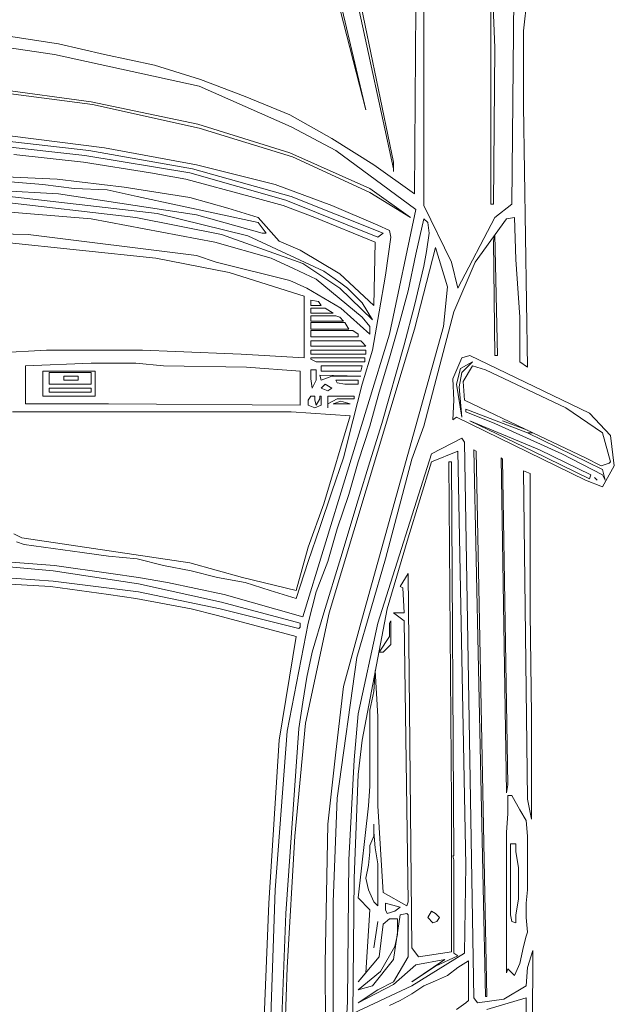
# Model space of a CAD drawing. Units: inches. Extents: x -36302355 to 648, y -221479757 to 75.
# Tile 9 of 37: x 209 to 227, y -484 to -455. Entities that reach past the tile are written whole.
import ezdxf

# ---------------------------------------------------------------- set-up
doc = ezdxf.new("R2010")
doc.units = ezdxf.units.IN
doc.header["$MEASUREMENT"] = 0
doc.layers.add('A-EQPM-VEHC', color=8, linetype='Continuous', lineweight=13)

msp = doc.modelspace()

# ---------------------------------------------------------------- linework, layer by layer
at = {"layer": 'A-EQPM-VEHC'}
for p, q in [((216.133, -443.293), (219.515, -457.606)), ((223.014, -446.517), (223.368, -455.758)), ((220.341, -459.375), (217.667, -447.067)), ((221.245, -447.264), (221.245, -460.477)), ((218.178, -448.798), (220.341, -459.178)), ((223.879, -460.437), (223.958, -452.847)), ((219.515, -457.606), (218.374, -453.163)), ((224.233, -455.246), (224.351, -454.146)), ((220.969, -460.122), (221.01, -454.539)), ((223.25, -460.437), (223.25, -454.618)), ((224.233, -457.489), (224.233, -455.246)), ((210.195, -455.955), (207.207, -455.522)), ((208.818, -455.404), (210.313, -455.639)), ((210.313, -455.639), (211.689, -455.955)), ((223.368, -455.758), (223.329, -460.437)), ((214.521, -456.899), (210.195, -455.955)), ((211.689, -455.955), (213.184, -456.269)), ((213.184, -456.269), (214.559, -456.701)), ((214.559, -456.701), (215.897, -457.213)), ((207.679, -456.976), (211.336, -457.448)), ((211.296, -457.369), (207.797, -456.899)), ((217.274, -458.117), (214.521, -456.899)), ((214.481, -458.038), (211.296, -457.369)), ((215.897, -457.213), (217.234, -457.764)), ((211.336, -457.448), (214.521, -458.157)), ((224.351, -465.313), (224.233, -457.489)), ((217.234, -457.764), (218.492, -458.471)), ((217.234, -458.903), (214.481, -458.038)), ((214.521, -458.157), (217.313, -459.022)), ((218.611, -458.826), (217.274, -458.117)), ((211.217, -458.826), (208.072, -458.471)), ((211.689, -458.747), (208.858, -458.392)), ((218.492, -458.471), (219.75, -459.257)), ((207.993, -458.629), (211.099, -458.982)), ((214.324, -459.375), (211.217, -458.826)), ((214.442, -459.257), (211.689, -458.747)), ((221.01, -460.594), (218.611, -458.826)), ((211.06, -459.178), (208.976, -458.943)), ((213.066, -459.494), (211.06, -459.178)), ((211.099, -458.982), (214.245, -459.494)), ((219.632, -459.966), (217.234, -458.903)), ((217.313, -459.022), (219.632, -460.084)), ((220.341, -459.178), (220.341, -459.454)), ((204.021, -459.375), (210.274, -459.691)), ((217.274, -460.201), (214.324, -459.375)), ((216.802, -459.847), (214.442, -459.257)), ((219.75, -459.257), (220.969, -460.122)), ((209.841, -459.847), (207.953, -459.691)), ((210.274, -459.691), (212.28, -459.926)), ((214.128, -459.691), (213.066, -459.494)), ((216.054, -460.201), (214.128, -459.691)), ((214.245, -459.494), (217.116, -460.319)), ((204.689, -459.808), (210.313, -460.122)), ((210.785, -459.966), (209.841, -459.847)), ((211.768, -460.005), (210.785, -459.966)), ((212.673, -460.201), (211.768, -460.005)), ((212.28, -459.926), (214.245, -460.24)), ((218.492, -460.477), (216.802, -459.847)), ((220.852, -460.831), (219.632, -459.966)), ((213.263, -460.712), (208.111, -460.122)), ((208.228, -460.319), (212.633, -460.831)), ((210.313, -460.122), (214.442, -460.752)), ((216.29, -460.988), (212.673, -460.201)), ((214.245, -460.24), (215.386, -460.556)), ((217.037, -460.477), (216.054, -460.201)), ((217.116, -460.319), (219.869, -461.421)), ((220.025, -461.302), (217.274, -460.201)), ((219.632, -460.084), (220.852, -460.831)), ((211.296, -460.87), (207.483, -460.556)), ((215.386, -460.556), (216.29, -460.831)), ((217.981, -460.831), (217.037, -460.477)), ((219.869, -461.066), (218.492, -460.477)), ((220.222, -464.33), (221.01, -460.594)), ((221.245, -460.477), (222.071, -462.167)), ((223.329, -460.437), (223.25, -460.437)), ((223.368, -460.831), (223.879, -460.437)), ((214.993, -461.577), (211.296, -460.87)), ((212.633, -460.831), (215.189, -461.342)), ((215.975, -461.381), (213.263, -460.712)), ((214.442, -460.752), (216.409, -461.302)), ((216.29, -460.831), (216.919, -461.538)), ((219.79, -461.577), (217.981, -460.831)), ((221.245, -460.87), (221.01, -461.932)), ((221.362, -460.988), (221.245, -460.87)), ((222.268, -462.954), (223.368, -460.831)), ((222.778, -462.167), (223.722, -460.87)), ((223.722, -460.87), (223.958, -460.831)), ((223.958, -460.831), (223.998, -462.089)), ((216.526, -461.302), (216.29, -460.988)), ((220.222, -461.224), (219.869, -461.066)), ((220.262, -461.421), (220.222, -461.224)), ((221.403, -461.302), (221.362, -460.988)), ((207.679, -461.302), (209.409, -461.342)), ((209.409, -461.342), (214.442, -461.97)), ((215.189, -461.342), (217.627, -462.207)), ((218.257, -462.442), (215.975, -461.381)), ((216.409, -461.302), (216.526, -461.302)), ((216.919, -461.538), (217.548, -461.814)), ((219.869, -461.421), (220.025, -461.302)), ((220.104, -462.561), (220.262, -461.421)), ((221.324, -461.853), (221.403, -461.302)), ((223.368, -461.342), (223.329, -461.538)), ((223.329, -461.538), (223.368, -464.96)), ((223.447, -464.96), (223.368, -461.342)), ((213.222, -462.049), (208.662, -461.577)), ((216.683, -462.049), (214.993, -461.577)), ((217.548, -461.814), (218.729, -462.521)), ((219.75, -463.465), (219.79, -461.577)), ((220.969, -464.172), (221.599, -461.735)), ((221.599, -461.735), (221.952, -462.914)), ((215.425, -462.482), (213.222, -462.049)), ((214.442, -461.97), (215.031, -462.167)), ((217.351, -462.365), (216.683, -462.049)), ((221.01, -461.932), (220.773, -463.032)), ((221.245, -462.286), (221.324, -461.853)), ((223.998, -462.089), (224.116, -463.82)), ((215.031, -462.167), (217.234, -462.718)), ((218.02, -462.679), (217.351, -462.365)), ((217.627, -462.207), (218.729, -462.954)), ((220.969, -463.465), (221.245, -462.286)), ((222.071, -462.167), (222.268, -462.954)), ((222.149, -463.662), (222.778, -462.167)), ((217.667, -463.19), (215.425, -462.482)), ((217.234, -462.718), (217.746, -462.954)), ((219.397, -463.82), (218.02, -462.679)), ((218.767, -462.797), (218.257, -462.442)), ((218.729, -462.521), (219.75, -463.465)), ((219.908, -463.662), (220.104, -462.561)), ((217.746, -462.954), (218.767, -463.544)), ((218.729, -462.954), (219.711, -463.898)), ((218.964, -462.954), (218.767, -462.797)), ((219.397, -463.386), (218.964, -462.954)), ((221.952, -462.914), (221.834, -464.095)), ((217.667, -465.037), (217.667, -463.19)), ((218.099, -463.348), (217.863, -463.307)), ((217.863, -463.307), (217.863, -463.465)), ((220.773, -463.032), (220.497, -464.055)), ((217.863, -463.465), (218.178, -463.465)), ((218.295, -463.544), (217.863, -463.544)), ((217.863, -463.544), (217.863, -463.7)), ((218.178, -463.465), (218.099, -463.348)), ((218.532, -463.7), (218.295, -463.544)), ((218.767, -463.544), (219.632, -464.33)), ((219.711, -463.898), (219.397, -463.386)), ((220.655, -464.644), (220.969, -463.465)), ((217.863, -463.7), (218.532, -463.7)), ((218.611, -463.779), (217.863, -463.779)), ((217.863, -463.779), (217.863, -463.937)), ((218.729, -463.82), (218.611, -463.779)), ((218.846, -463.937), (218.729, -463.82)), ((219.632, -464.095), (219.397, -463.82)), ((219.711, -464.802), (219.908, -463.662)), ((221.245, -467.083), (222.149, -463.662)), ((224.116, -463.82), (224.116, -465.157)), ((217.863, -463.937), (218.846, -463.937)), ((218.885, -463.976), (217.863, -463.976)), ((217.863, -463.976), (217.863, -464.172)), ((217.863, -464.172), (219.004, -464.172)), ((218.413, -472.667), (220.969, -464.172)), ((219.004, -464.172), (218.885, -463.976)), ((221.834, -464.095), (219.357, -472.981)), ((219.632, -464.33), (219.632, -464.095)), ((220.497, -464.055), (220.222, -465.037)), ((217.627, -472.784), (220.222, -464.33)), ((219.122, -464.213), (217.863, -464.213)), ((217.863, -464.213), (217.863, -464.409)), ((217.863, -464.409), (219.279, -464.409)), ((219.279, -464.33), (219.122, -464.213)), ((219.279, -464.409), (219.279, -464.33)), ((219.357, -464.527), (217.863, -464.527)), ((217.863, -464.527), (217.863, -464.685)), ((217.863, -464.685), (219.515, -464.685)), ((219.397, -464.565), (219.357, -464.527)), ((219.515, -464.685), (219.397, -464.565)), ((219.987, -467.004), (220.655, -464.644)), ((207.993, -464.92), (209.959, -464.802)), ((209.959, -464.802), (212.829, -464.802)), ((212.829, -464.802), (213.814, -464.841)), ((213.814, -464.841), (215.779, -464.92)), ((215.779, -464.92), (217.667, -465.037)), ((219.515, -464.802), (217.863, -464.802)), ((217.863, -464.802), (217.863, -464.92)), ((217.863, -464.92), (219.515, -464.92)), ((219.476, -465.037), (217.863, -465.037)), ((217.863, -465.037), (217.863, -465.078)), ((217.863, -465.078), (218.02, -465.157)), ((219.397, -465.825), (219.711, -464.802)), ((219.476, -465.157), (219.476, -465.037)), ((219.515, -464.92), (219.515, -464.802)), ((220.222, -465.037), (219.908, -466.06)), ((222.385, -465.037), (222.11, -465.667)), ((222.621, -464.96), (222.385, -465.037)), ((226.2, -466.69), (222.621, -464.96)), ((223.368, -464.96), (223.447, -464.96)), ((211.296, -465.195), (209.33, -465.274)), ((209.33, -465.274), (209.33, -466.415)), ((212.633, -465.195), (211.296, -465.195)), ((213.459, -465.274), (212.633, -465.195)), ((215.937, -465.313), (213.459, -465.274)), ((217.548, -465.431), (215.937, -465.313)), ((218.02, -465.157), (219.476, -465.157)), ((219.397, -465.274), (218.178, -465.274)), ((218.178, -465.274), (218.178, -465.431)), ((219.357, -465.431), (219.397, -465.274)), ((222.345, -465.353), (222.228, -465.825)), ((222.7, -465.157), (222.345, -465.353)), ((222.385, -465.471), (222.7, -465.157)), ((222.7, -465.274), (222.424, -465.746)), ((223.093, -465.392), (222.7, -465.274)), ((224.116, -465.157), (224.351, -465.313)), ((211.415, -465.431), (209.841, -465.431)), ((209.841, -465.431), (209.841, -466.178)), ((211.296, -465.471), (210.038, -465.471)), ((210.038, -465.471), (210.038, -465.825)), ((210.903, -465.588), (210.471, -465.588)), ((210.471, -465.588), (210.471, -465.706)), ((210.903, -465.706), (210.903, -465.588)), ((211.296, -465.825), (211.296, -465.471)), ((211.415, -466.178), (211.415, -465.431)), ((217.548, -466.453), (217.548, -465.431)), ((218.02, -465.392), (217.863, -465.392)), ((217.863, -465.392), (217.863, -465.667)), ((217.863, -465.667), (217.902, -465.943)), ((218.02, -465.706), (218.02, -465.392)), ((219.357, -465.588), (218.139, -465.55)), ((218.139, -465.55), (218.178, -465.706)), ((218.178, -465.431), (219.357, -465.431)), ((218.178, -465.706), (218.492, -465.588)), ((218.492, -465.588), (219.357, -465.588)), ((222.11, -465.667), (222.149, -466.297)), ((222.306, -465.903), (222.385, -465.471)), ((225.491, -466.532), (223.093, -465.392)), ((210.038, -465.825), (211.296, -465.825)), ((211.296, -465.943), (210.038, -465.943)), ((210.038, -465.943), (210.038, -466.06)), ((210.471, -465.706), (210.903, -465.706)), ((211.296, -466.06), (211.296, -465.943)), ((217.902, -465.943), (218.02, -465.706)), ((218.295, -465.825), (218.178, -465.943)), ((218.178, -465.943), (218.374, -466.022)), ((218.492, -465.943), (218.295, -465.825)), ((218.374, -466.022), (218.492, -465.943)), ((219.279, -465.706), (218.611, -465.706)), ((218.611, -465.706), (218.65, -465.785)), ((218.65, -465.785), (218.885, -465.825)), ((218.885, -465.825), (219.279, -465.825)), ((219.122, -466.925), (219.397, -465.825)), ((219.279, -465.825), (219.279, -465.706)), ((222.228, -465.825), (222.385, -466.808)), ((222.385, -466.808), (222.306, -465.903)), ((222.424, -465.746), (222.464, -466.297)), ((209.841, -466.178), (211.415, -466.178)), ((210.038, -466.06), (211.296, -466.06)), ((217.863, -466.178), (217.785, -466.297)), ((217.981, -466.178), (217.863, -466.178)), ((217.981, -466.297), (217.981, -466.178)), ((218.139, -466.257), (218.02, -466.453)), ((218.178, -466.178), (218.139, -466.178)), ((218.139, -466.178), (218.139, -466.257)), ((218.178, -466.453), (218.178, -466.178)), ((219.16, -466.178), (218.374, -466.178)), ((218.374, -466.178), (218.374, -466.532)), ((218.374, -466.415), (218.65, -466.257)), ((218.65, -466.257), (219.16, -466.257)), ((219.16, -466.257), (219.16, -466.178)), ((219.908, -466.06), (219.632, -467.083)), ((209.33, -466.415), (211.808, -466.415)), ((211.808, -466.415), (217.548, -466.453)), ((217.785, -466.297), (217.785, -466.453)), ((217.785, -466.453), (217.981, -466.532)), ((218.02, -466.453), (217.981, -466.297)), ((217.981, -466.532), (218.178, -466.453)), ((218.767, -466.336), (218.532, -466.415)), ((218.532, -466.415), (219.043, -466.415)), ((219.043, -466.415), (218.767, -466.336)), ((222.149, -466.297), (222.11, -466.887)), ((222.464, -466.297), (224.509, -467.28)), ((226.593, -467.28), (225.491, -466.532)), ((217.274, -466.65), (208.937, -466.65)), ((219.043, -466.768), (217.274, -466.65)), ((218.257, -469.403), (219.043, -466.768)), ((222.11, -466.887), (222.228, -466.808)), ((222.228, -466.808), (226.081, -468.696)), ((224.351, -467.28), (222.503, -466.571)), ((222.503, -466.571), (222.503, -466.65)), ((222.503, -466.65), (223.368, -467.004)), ((226.828, -467.359), (226.2, -466.69)), ((218.846, -468.027), (219.122, -466.925)), ((219.632, -467.083), (219.279, -468.145)), ((219.632, -468.145), (219.987, -467.004)), ((220.89, -468.066), (221.245, -467.083)), ((222.621, -466.925), (224.509, -467.831)), ((224.705, -467.791), (222.621, -466.925)), ((223.368, -467.004), (225.374, -467.908)), ((223.605, -466.925), (224.351, -467.201)), ((222.385, -467.436), (221.48, -467.908)), ((222.464, -467.555), (222.385, -467.436)), ((226.593, -468.38), (224.351, -467.28)), ((224.351, -467.28), (224.509, -467.28)), ((224.509, -467.28), (226.081, -468.027)), ((226.828, -468.145), (226.593, -467.28)), ((226.946, -468.263), (226.828, -467.359)), ((222.74, -484.188), (222.464, -467.555)), ((218.492, -469.049), (218.846, -468.027)), ((221.48, -467.908), (219.869, -472.981)), ((222.268, -467.831), (221.48, -468.145)), ((222.503, -480.217), (222.268, -467.831)), ((222.817, -467.831), (222.74, -467.791)), ((222.74, -467.791), (223.093, -484.15)), ((223.133, -484.15), (222.817, -467.831)), ((223.605, -468.066), (223.565, -468.027)), ((223.565, -468.027), (223.722, -478.054)), ((224.509, -467.831), (226.2, -468.656)), ((226.239, -468.538), (224.705, -467.791)), ((225.374, -467.908), (226.593, -468.538)), ((226.081, -468.027), (226.553, -468.263)), ((219.279, -468.145), (219.004, -469.128)), ((219.279, -469.285), (219.632, -468.145)), ((220.104, -471.054), (220.89, -468.066)), ((221.48, -468.145), (220.773, -470.426)), ((222.071, -468.145), (221.992, -468.145)), ((221.992, -468.145), (222.071, -478.368)), ((222.149, -479.942), (222.071, -468.145)), ((223.761, -477.819), (223.605, -468.066)), ((226.553, -468.263), (226.79, -468.184)), ((226.593, -468.892), (226.946, -468.263)), ((226.79, -468.184), (226.828, -468.145)), ((224.43, -468.498), (224.233, -468.42)), ((224.233, -468.42), (224.351, -478.25)), ((224.43, -472.667), (224.43, -468.498)), ((226.2, -468.656), (226.239, -468.538)), ((226.356, -468.617), (226.435, -468.696)), ((226.672, -468.696), (226.593, -468.38)), ((226.593, -468.538), (226.672, -468.696)), ((226.081, -468.696), (226.593, -468.892)), ((218.139, -470.11), (218.492, -469.049)), ((219.004, -469.128), (218.65, -470.151)), ((217.785, -470.7), (218.257, -469.403)), ((218.767, -471.016), (219.279, -469.285)), ((208.976, -470.307), (209.213, -470.426)), ((217.785, -471.133), (218.139, -470.11)), ((218.65, -470.151), (218.374, -471.133)), ((209.055, -470.544), (209.29, -470.623)), ((209.213, -470.426), (214.245, -471.172)), ((209.29, -470.623), (211.02, -470.858)), ((220.773, -470.426), (220.145, -472.549)), ((211.02, -470.858), (211.808, -470.975)), ((211.808, -470.975), (212.673, -471.054)), ((217.43, -471.998), (217.785, -470.7)), ((207.56, -471.054), (210.195, -471.251)), ((210.155, -471.409), (207.56, -471.172)), ((210.195, -471.251), (211.885, -471.488)), ((212.673, -471.054), (213.459, -471.251)), ((213.459, -471.251), (214.284, -471.409)), ((214.245, -471.172), (215.818, -471.605)), ((217.43, -472.234), (217.785, -471.133)), ((218.374, -471.133), (218.02, -472.037)), ((218.257, -472.667), (218.767, -471.016)), ((219.239, -474.004), (220.104, -471.054)), ((207.56, -471.526), (210.155, -471.723)), ((212.712, -471.802), (210.155, -471.409)), ((211.885, -471.488), (212.712, -471.605)), ((214.284, -471.409), (215.072, -471.605)), ((220.773, -471.488), (220.538, -471.881)), ((220.89, -482.693), (220.773, -471.488)), ((210.078, -471.881), (207.483, -471.723)), ((210.155, -471.723), (212.712, -472.037)), ((212.712, -471.605), (213.577, -471.763)), ((215.189, -472.353), (212.712, -471.802)), ((213.577, -471.763), (215.268, -472.116)), ((215.072, -471.605), (215.897, -471.763)), ((215.818, -471.605), (217.43, -471.998)), ((215.897, -471.763), (216.644, -471.998)), ((211.808, -472.116), (210.078, -471.881)), ((212.633, -472.234), (211.808, -472.116)), ((212.712, -472.037), (215.149, -472.549)), ((215.268, -472.116), (217.627, -472.784)), ((216.644, -471.998), (217.43, -472.234)), ((218.02, -472.037), (217.785, -472.981)), ((220.538, -471.881), (220.615, -471.919)), ((220.615, -471.919), (220.655, -472.667)), ((214.284, -472.549), (212.633, -472.234)), ((217.548, -472.981), (215.189, -472.353)), ((215.072, -472.746), (214.284, -472.549)), ((215.149, -472.549), (217.509, -473.139)), ((217.706, -475.969), (218.413, -472.667)), ((217.902, -473.846), (218.257, -472.667)), ((220.145, -472.549), (219.397, -476.482)), ((220.655, -472.667), (220.341, -472.667)), ((220.341, -472.667), (220.655, -472.902)), ((224.47, -475.734), (224.43, -472.667)), ((217.43, -473.374), (215.072, -472.746)), ((217.785, -472.981), (217.155, -476.206)), ((217.548, -473.099), (217.548, -472.981)), ((219.357, -472.981), (218.846, -474.869)), ((219.869, -472.981), (219.279, -475.695)), ((220.262, -472.902), (220.222, -472.981)), ((220.222, -472.981), (220.222, -473.374)), ((220.262, -473.611), (220.262, -472.902)), ((220.655, -472.902), (220.773, -481.318)), ((217.509, -473.139), (217.548, -473.099)), ((216.919, -476.482), (217.43, -473.374)), ((220.222, -473.374), (219.908, -473.846)), ((220.025, -473.846), (220.262, -473.611)), ((217.746, -474.594), (217.902, -473.846)), ((219.908, -473.846), (220.025, -473.846)), ((218.65, -478.212), (219.239, -474.004)), ((219.79, -474.397), (219.75, -475.027)), ((219.869, -475.773), (219.79, -474.397)), ((217.627, -475.341), (217.746, -474.594)), ((218.846, -474.869), (218.611, -476.834)), ((219.75, -475.027), (219.632, -475.576)), ((217.509, -476.127), (217.627, -475.341)), ((219.632, -475.576), (219.632, -477.857)), ((217.391, -479.352), (217.706, -475.969)), ((219.279, -475.695), (219.16, -477.071)), ((219.869, -478.447), (219.869, -475.773)), ((224.47, -478.84), (224.47, -475.734)), ((217.155, -476.206), (216.802, -480.963)), ((217.116, -481.672), (217.509, -476.127)), ((216.605, -481.358), (216.919, -476.482)), ((219.397, -476.482), (219.279, -477.503)), ((218.611, -476.834), (218.374, -478.998)), ((219.16, -477.071), (219.004, -480.059)), ((219.279, -477.503), (219.16, -480.61)), ((219.632, -477.857), (219.594, -478.447)), ((223.722, -478.054), (223.761, -477.819)), ((218.532, -481.318), (218.65, -478.212)), ((223.879, -478.133), (223.761, -478.133)), ((223.761, -478.133), (223.761, -478.684)), ((224.116, -478.565), (223.879, -478.133)), ((224.351, -478.25), (224.47, -478.84)), ((219.594, -478.447), (219.279, -481.2)), ((220.025, -481.042), (219.869, -478.447)), ((222.071, -478.368), (222.071, -482.813)), ((224.312, -478.88), (224.116, -478.565)), ((223.761, -478.684), (223.722, -479.233)), ((224.351, -479.352), (224.312, -478.88)), ((218.374, -478.998), (218.295, -483.165)), ((219.75, -478.998), (219.75, -479.352)), ((217.155, -483.285), (217.391, -479.352)), ((219.75, -479.352), (219.632, -479.628)), ((219.79, -479.705), (219.75, -479.233)), ((223.722, -479.233), (223.722, -483.441)), ((224.351, -480.963), (224.351, -479.352)), ((219.632, -479.628), (219.632, -479.824)), ((219.869, -480.177), (219.79, -479.705)), ((223.998, -479.587), (223.84, -479.587)), ((223.84, -479.587), (223.84, -481.711)), ((223.998, -479.824), (223.998, -479.587)), ((219.004, -480.059), (218.964, -484.306)), ((219.632, -479.824), (219.594, -480.217)), ((222.149, -480.059), (222.11, -479.942)), ((222.11, -479.942), (222.149, -479.942)), ((222.149, -482.851), (222.149, -480.059)), ((224.077, -480.295), (223.998, -479.824)), ((219.594, -480.217), (219.515, -480.61)), ((219.869, -481.435), (219.869, -480.177)), ((222.464, -482.851), (222.503, -480.217)), ((224.077, -481.239), (224.077, -480.295)), ((219.16, -480.61), (219.122, -484.66)), ((219.515, -480.61), (219.594, -480.963)), ((216.802, -480.963), (215.937, -505.148)), ((219.594, -480.963), (219.75, -481.318)), ((224.312, -481.358), (224.351, -480.963)), ((219.279, -481.2), (219.632, -481.554)), ((220.734, -481.435), (220.025, -481.042)), ((223.998, -481.711), (224.077, -481.239)), ((216.409, -486.194), (216.605, -481.358)), ((218.532, -485.643), (218.532, -481.318)), ((219.632, -481.554), (219.515, -483.441)), ((219.75, -481.318), (219.869, -481.435)), ((220.538, -481.475), (220.104, -481.358)), ((220.104, -481.358), (220.104, -481.554)), ((220.104, -481.554), (220.145, -481.672)), ((220.38, -481.593), (220.538, -481.475)), ((220.773, -481.318), (220.734, -481.435)), ((224.312, -481.79), (224.312, -481.358)), ((216.251, -505.148), (217.116, -481.672)), ((220.025, -481.986), (220.222, -481.828)), ((220.145, -481.672), (220.38, -481.593)), ((220.222, -481.828), (220.459, -481.828)), ((220.341, -483.048), (220.538, -481.711)), ((220.459, -481.828), (220.459, -482.3)), ((220.538, -481.711), (220.734, -481.672)), ((220.734, -481.672), (220.773, -481.711)), ((220.773, -481.711), (220.773, -482.969)), ((221.48, -481.593), (221.362, -481.79)), ((221.362, -481.79), (221.52, -481.947)), ((221.599, -481.672), (221.48, -481.593)), ((221.717, -481.79), (221.599, -481.672)), ((221.638, -481.907), (221.717, -481.79)), ((223.84, -481.711), (223.879, -481.907)), ((223.998, -481.947), (223.998, -481.711)), ((224.351, -482.223), (224.312, -481.79)), ((219.75, -482.693), (219.869, -481.907)), ((219.908, -482.969), (220.025, -481.986)), ((221.52, -481.947), (221.638, -481.907)), ((223.879, -481.907), (223.998, -481.947)), ((220.459, -482.3), (220.38, -482.655)), ((224.233, -482.655), (224.312, -482.341)), ((224.312, -482.341), (224.351, -482.223)), ((220.38, -482.655), (219.946, -483.402)), ((221.087, -482.969), (220.89, -482.693)), ((224.116, -483.165), (224.233, -482.655)), ((219.279, -483.716), (219.908, -482.969)), ((219.711, -483.834), (220.341, -483.048)), ((220.773, -482.969), (220.341, -483.716)), ((220.89, -483.834), (222.464, -482.851)), ((221.875, -483.048), (220.89, -483.716)), ((221.01, -483.206), (221.875, -483.048)), ((222.071, -482.813), (221.087, -482.969)), ((221.599, -483.244), (222.268, -482.93)), ((222.268, -482.93), (222.149, -482.851)), ((224.509, -482.772), (224.351, -483.285)), ((224.47, -492.957), (224.509, -482.772)), ((216.486, -504.439), (217.155, -483.285)), ((218.295, -483.165), (218.374, -494.452)), ((220.341, -483.795), (221.01, -483.206)), ((220.89, -483.716), (221.599, -483.244)), ((221.952, -483.52), (222.268, -483.285)), ((222.268, -483.285), (222.582, -483.088)), ((222.582, -483.088), (222.582, -484.267)), ((223.722, -483.441), (223.761, -483.323)), ((223.761, -483.323), (223.958, -483.52)), ((223.958, -483.52), (224.116, -483.165)), ((224.351, -483.285), (224.312, -483.834)), ((219.946, -483.402), (219.279, -483.953)), ((219.515, -483.441), (219.279, -483.716)), ((221.599, -483.678), (221.952, -483.52)), ((219.122, -484.66), (220.89, -483.834)), ((219.279, -484.346), (220.341, -483.795)), ((219.279, -483.953), (219.711, -483.834)), ((220.341, -483.716), (219.869, -483.953)), ((220.89, -484.071), (221.245, -483.834)), ((221.245, -483.834), (221.599, -483.678)), ((224.312, -483.834), (223.644, -484.227)), ((219.869, -483.953), (219.279, -484.346)), ((220.538, -484.267), (220.89, -484.071)), ((222.857, -484.346), (222.74, -484.188)), ((223.644, -484.227), (222.857, -484.346)), ((223.093, -484.15), (223.133, -484.15)), ((223.133, -484.543), (224.312, -484.188)), ((224.312, -484.188), (224.194, -498.226)), ((218.964, -484.306), (218.885, -485.643)), ((220.222, -484.425), (220.538, -484.267)), ((222.503, -484.346), (222.228, -484.543)), ((222.582, -484.267), (222.503, -484.346))]:
    msp.add_line(p, q, dxfattribs=at)

doc.saveas('drawing.dxf')
